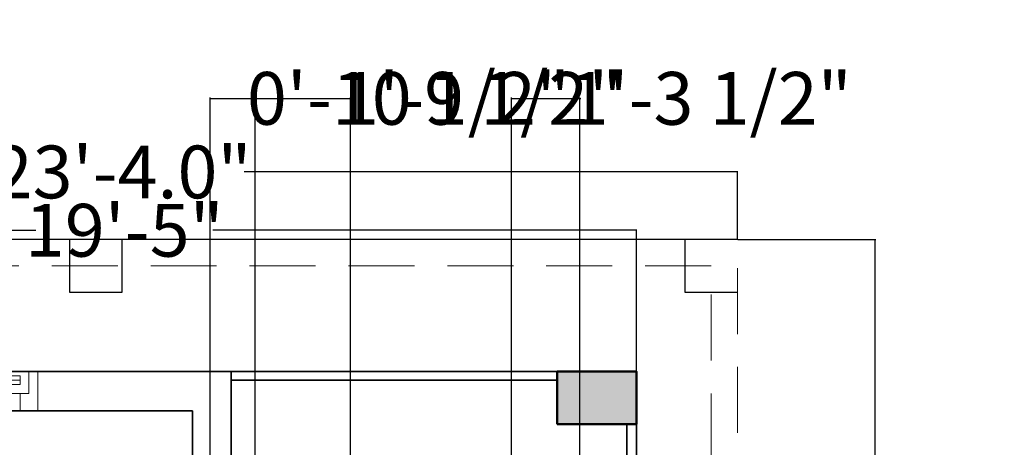
# Model space of a CAD drawing. Units: inches. Extents: x 1063 to 2718, y 423 to 1923.
# Tile 6 of 7: x 1268 to 1492, y 1038 to 1135. Entities that reach past the tile are written whole.
import ezdxf

# ---------------------------------------------------------------- set-up
doc = ezdxf.new("R2010")
doc.units = ezdxf.units.IN
doc.header["$LTSCALE"] = 6
doc.header["$MEASUREMENT"] = 0
doc.linetypes.add('HIDDEN', pattern=[0.375, 0.25, -0.125])
for name, color, linetype, lineweight in [('A-ANNO-DIMS', 2, 'Continuous', 18), ('A-COLS', 7, 'Continuous', 50), ('A-COLS-PATT', 252, 'Continuous', 13), ('A-GLAZ', 4, 'Continuous', 18), ('A-WALL', 7, 'Continuous', 35), ('C-PROP', 7, 'Continuous', 25), ('C-PROP-HIDN', 7, 'HIDDEN', 18)]:
    doc.layers.add(name, color=color, linetype=linetype, lineweight=lineweight)
doc.styles.get("Standard").update_dxf_attribs({"font": 'arial.ttf'})
doc.dimstyles.get("Standard").update_dxf_attribs({"dimtxt": 12, "dimasz": 0.18, "dimexe": 0.18, "dimexo": 0.0625, "dimgap": 0.09, "dimtad": 0, "dimtih": 1, "dimtoh": 1, "dimdec": 1, "dimzin": 0, "dimdsep": 46, "dimlunit": 3, "dimtxsty": 'Standard', "dimcen": 0.09, "dimadec": 0, "dimazin": 0, "dimtfac": 1, "dimtdec": 1, "dimtofl": 0, "dimtmove": 0, "dimatfit": 3, "dimfxl": 1, "dimtolj": 1, "dimtzin": 0, "dimarcsym": 0})

# ---------------------------------------------------------------- blocks, each defined once
blk = doc.blocks.new('*D5')
at = {"layer": 'A-ANNO-DIMS', "color": 0, "lineweight": -2, "ltscale": 6, "transparency": 16777216}
for p, q in [((1430.99, 1085.12), (1462.35, 1085.12)), ((1462.17, 1084.94), (1462.17, 1024.34)), ((1462.17, 951.3), (1462.17, 1011.9)), ((1430.99, 951.12), (1462.35, 951.12))]:
    blk.add_line(p, q, dxfattribs=at)
at = {"layer": 'A-ANNO-DIMS', "color": 0, "ltscale": 6, "transparency": 16777216}
for points in [[(1462.14, 1084.94), (1462.2, 1084.94), (1462.17, 1085.12)], [(1462.14, 951.3), (1462.2, 951.3), (1462.17, 951.12)]]:
    blk.add_solid(points, dxfattribs=at)
at = {"layer": 'Defpoints', "color": 0, "ltscale": 6, "transparency": 16777216}
for p in [(1430.93, 1085.12), (1462.17, 1085.12), (1430.93, 951.12)]:
    blk.add_point(p, dxfattribs=at)
at = {"layer": 'A-ANNO-DIMS', "color": 0, "ltscale": 6, "transparency": 16777216, "insert": (1462.17, 1018.12), "char_height": 12, "attachment_point": 5}
blk.add_mtext('\\A1;11\'-2.0"', dxfattribs=at)
blk = doc.blocks.new('*D6')
at = {"layer": 'A-ANNO-DIMS', "color": 0, "lineweight": -2, "ltscale": 6, "transparency": 16777216}
for p, q in [((1150.93, 1085.18), (1150.93, 1100.66)), ((1151.11, 1100.48), (1263.13, 1100.48)), ((1430.75, 1100.48), (1318.72, 1100.48)), ((1430.93, 1085.18), (1430.93, 1100.66))]:
    blk.add_line(p, q, dxfattribs=at)
at = {"layer": 'A-ANNO-DIMS', "color": 0, "ltscale": 6, "transparency": 16777216}
for points in [[(1151.11, 1100.51), (1151.11, 1100.45), (1150.93, 1100.48)], [(1430.75, 1100.51), (1430.75, 1100.45), (1430.93, 1100.48)]]:
    blk.add_solid(points, dxfattribs=at)
at = {"layer": 'Defpoints', "color": 0, "ltscale": 6, "transparency": 16777216}
for p in [(1430.93, 1100.48), (1150.93, 1085.12), (1430.93, 1085.12)]:
    blk.add_point(p, dxfattribs=at)
at = {"layer": 'A-ANNO-DIMS', "color": 0, "ltscale": 6, "transparency": 16777216, "insert": (1290.93, 1100.48), "char_height": 12, "attachment_point": 5}
blk.add_mtext('\\A1;23\'-4.0"', dxfattribs=at)
blk = doc.blocks.new('WIN-48-SLIDING')
at = {"ltscale": 6}
for p, q in [((0, 9), (4, 9)), ((4, 9), (4, 5)), ((48, 9), (44, 9)), ((44, 9), (44, 5)), ((4, 5), (2, 5)), ((2, 5), (2, 0)), ((4, 5), (44, 5)), ((4, 5), (6, 5)), ((6, 5), (6, 3)), ((44, 5), (42, 5)), ((42, 5), (42, 3)), ((44, 5), (46, 5)), ((46, 5), (46, 0)), ((6, 3), (4, 3)), ((4, 3), (4, 1)), ((42, 3), (44, 3)), ((44, 3), (44, 1)), ((4, 2), (44, 2)), ((4, 1), (6, 1)), ((6, 1), (6, 0)), ((44, 1), (42, 1)), ((42, 1), (42, 0)), ((48, 0), (0, 0)), ((2, 0), (46, 0))]:
    blk.add_line(p, q, dxfattribs=at)
blk.add_lwpolyline([(48, 0), (48, 9), (0, 9), (0, 0)], dxfattribs=at)
blk = doc.blocks.new('COLUMN-18X12')
blk.add_lwpolyline([(0, 0), (18, 0), (18, 12), (0, 12)], close=True)
blk = doc.blocks.new('PIER-12X12-CORNER')
blk.add_lwpolyline([(0, 0), (12, 0), (12, 12)])
blk = doc.blocks.new('PIER-12X12-INLINE')
blk.add_lwpolyline([(0, 0), (12, 0), (12, 12), (0, 12)])
blk = doc.blocks.new('*D44')
at = {"layer": 'A-ANNO-DIMS', "color": 0, "lineweight": -2, "ltscale": 6, "transparency": 16777216}
for p, q in [((1174.93, 1055.18), (1174.93, 1087.4)), ((1175.11, 1087.22), (1271.29, 1087.22)), ((1407.75, 1087.22), (1311.56, 1087.22)), ((1407.93, 1055.18), (1407.93, 1087.4))]:
    blk.add_line(p, q, dxfattribs=at)
at = {"layer": 'A-ANNO-DIMS', "color": 0, "ltscale": 6, "transparency": 16777216}
for points in [[(1175.11, 1087.25), (1175.11, 1087.19), (1174.93, 1087.22)], [(1407.75, 1087.25), (1407.75, 1087.19), (1407.93, 1087.22)]]:
    blk.add_solid(points, dxfattribs=at)
at = {"layer": 'Defpoints', "color": 0, "ltscale": 6, "transparency": 16777216}
for p in [(1407.93, 1087.22), (1174.93, 1055.12), (1407.93, 1055.12)]:
    blk.add_point(p, dxfattribs=at)
at = {"layer": 'A-ANNO-DIMS', "color": 0, "ltscale": 6, "transparency": 16777216, "insert": (1291.43, 1087.22), "char_height": 12, "attachment_point": 5}
blk.add_mtext('\\A1;19\'-5"', dxfattribs=at)
blk = doc.blocks.new('*D60')
at = {"layer": 'A-ANNO-DIMS', "color": 0, "lineweight": -2, "ltscale": 6, "transparency": 16777216}
for p, q in [((1321.21, 974.62), (1321.21, 1117.4)), ((1321.39, 1117.22), (1342.7, 1117.22)), ((1342.88, 974.62), (1342.88, 1117.4)), ((1342.88, 1117.22), (1343.06, 1117.22))]:
    blk.add_line(p, q, dxfattribs=at)
at = {"layer": 'A-ANNO-DIMS', "color": 0, "ltscale": 6, "transparency": 16777216}
for points in [[(1321.39, 1117.25), (1321.39, 1117.19), (1321.21, 1117.22)], [(1342.7, 1117.25), (1342.7, 1117.19), (1342.88, 1117.22)]]:
    blk.add_solid(points, dxfattribs=at)
at = {"layer": 'Defpoints', "color": 0, "ltscale": 6, "transparency": 16777216}
for p in [(1342.88, 1117.22), (1321.21, 974.55), (1342.88, 974.55)]:
    blk.add_point(p, dxfattribs=at)
at = {"layer": 'A-ANNO-DIMS', "color": 0, "ltscale": 6, "transparency": 16777216, "insert": (1372.52, 1117.22), "char_height": 12, "attachment_point": 5}
blk.add_mtext('\\A1;1\'-9 1/2"', dxfattribs=at)
blk = doc.blocks.new('*D62')
at = {"layer": 'A-ANNO-DIMS', "color": 0, "lineweight": -2, "ltscale": 6, "transparency": 16777216}
for p, q in [((1379.5, 974.73), (1379.5, 1117.4)), ((1379.68, 1117.22), (1394.9, 1117.22)), ((1395.08, 974.73), (1395.08, 1117.4)), ((1395.08, 1117.22), (1395.26, 1117.22))]:
    blk.add_line(p, q, dxfattribs=at)
at = {"layer": 'A-ANNO-DIMS', "color": 0, "ltscale": 6, "transparency": 16777216}
for points in [[(1379.68, 1117.25), (1379.68, 1117.19), (1379.5, 1117.22)], [(1394.9, 1117.25), (1394.9, 1117.19), (1395.08, 1117.22)]]:
    blk.add_solid(points, dxfattribs=at)
at = {"layer": 'Defpoints', "color": 0, "ltscale": 6, "transparency": 16777216}
for p in [(1395.08, 1117.22), (1379.5, 974.67), (1395.08, 974.67)]:
    blk.add_point(p, dxfattribs=at)
at = {"layer": 'A-ANNO-DIMS', "color": 0, "ltscale": 6, "transparency": 16777216, "insert": (1424.71, 1117.22), "char_height": 12, "attachment_point": 5}
blk.add_mtext('\\A1;1\'-3 1/2"', dxfattribs=at)
blk = doc.blocks.new('*D64')
at = {"layer": 'A-ANNO-DIMS', "color": 0, "lineweight": -2, "ltscale": 6, "transparency": 16777216}
for p, q in [((1310.93, 978.18), (1310.93, 1117.4)), ((1311.11, 1117.22), (1321.03, 1117.22)), ((1321.21, 974.62), (1321.21, 1117.4)), ((1321.21, 1117.22), (1321.39, 1117.22))]:
    blk.add_line(p, q, dxfattribs=at)
at = {"layer": 'A-ANNO-DIMS', "color": 0, "ltscale": 6, "transparency": 16777216}
for points in [[(1311.11, 1117.25), (1311.11, 1117.19), (1310.93, 1117.22)], [(1321.03, 1117.25), (1321.03, 1117.19), (1321.21, 1117.22)]]:
    blk.add_solid(points, dxfattribs=at)
at = {"layer": 'Defpoints', "color": 0, "ltscale": 6, "transparency": 16777216}
for p in [(1321.21, 1117.22), (1310.93, 978.12), (1321.21, 974.55)]:
    blk.add_point(p, dxfattribs=at)
at = {"layer": 'A-ANNO-DIMS', "color": 0, "ltscale": 6, "transparency": 16777216, "insert": (1356.07, 1117.22), "char_height": 12, "attachment_point": 5}
blk.add_mtext('\\A1;0\'-10 1/2"', dxfattribs=at)

msp = doc.modelspace()

# ---------------------------------------------------------------- hatches: boundary and pattern name
at = {"layer": 'A-COLS-PATT', "ltscale": 6}
h = msp.add_hatch(color=256, dxfattribs=at)
h.dxf.hatch_style = 1
h.paths.add_polyline_path([(1192.93, 603.12), (1174.93, 603.12), (1174.93, 591.12), (1192.93, 591.12)])
h.paths.add_polyline_path([(1407.93, 603.12), (1389.93, 603.12), (1389.93, 591.12), (1407.93, 591.12)])
h.paths.add_polyline_path([(1192.93, 756.12), (1174.93, 756.12), (1174.93, 744.12), (1192.93, 744.12)])
h.paths.add_polyline_path([(1407.93, 761.11), (1389.93, 761.11), (1389.93, 749.11), (1407.93, 749.11)])
h.paths.add_polyline_path([(1455.93, 761.11), (1437.93, 761.11), (1437.93, 749.11), (1455.93, 749.11)])
h.paths.add_polyline_path([(1455.93, 910.12), (1437.93, 910.12), (1437.93, 898.12), (1455.93, 898.12)])
h.paths.add_polyline_path([(1407.93, 910.12), (1389.93, 910.12), (1389.93, 898.12), (1407.93, 898.12)])
h.paths.add_polyline_path([(1192.93, 910.12), (1174.93, 910.12), (1174.93, 898.12), (1192.93, 898.12)])
h.paths.add_polyline_path([(1192.93, 1055.12), (1174.93, 1055.12), (1174.93, 1043.12), (1192.93, 1043.12)])
h.paths.add_polyline_path([(1407.93, 1055.12), (1389.93, 1055.12), (1389.93, 1043.12), (1407.93, 1043.12)])

# ---------------------------------------------------------------- linework, layer by layer
at = {"layer": 'A-WALL'}
for p, q in [((1407.93, 1055.12), (1174.93, 1055.12)), ((1315.75, 1055.12), (1315.75, 987.12)), ((1315.75, 1053.12), (1389.93, 1053.12)), ((1306.93, 1046.12), (1192.93, 1046.12)), ((1306.93, 1046.12), (1306.93, 902.12)), ((1405.75, 1043.12), (1405.75, 987.12))]:
    msp.add_line(p, q, dxfattribs=at)
at = {"layer": 'A-WALL', "ltscale": 6}
msp.add_line((1407.93, 1055.12), (1407.93, 591.12), dxfattribs=at)
at = {"layer": 'C-PROP'}
msp.add_line((1430.93, 1085.12), (1150.93, 1085.12), dxfattribs=at)
at = {"layer": 'C-PROP-HIDN', "ltscale": 10}
for p, q in [((1430.93, 951.12), (1430.93, 1085.12)), ((1424.93, 1079.12), (1156.93, 1079.12)), ((1424.93, 945.12), (1424.93, 1079.12))]:
    msp.add_line(p, q, dxfattribs=at)

# ---------------------------------------------------------------- block references
at = {"layer": 'A-COLS'}
msp.add_blockref('COLUMN-18X12', (1389.93, 1043.12), dxfattribs=at)
at = {"layer": 'A-GLAZ', "rotation": 180}
msp.add_blockref('WIN-48-SLIDING', (1271.72, 1055.12), dxfattribs=at)
at = {"layer": 'C-PROP', "rotation": 270}
for name, p in [('PIER-12X12-INLINE', (1278.93, 1085.12)), ('PIER-12X12-CORNER', (1418.93, 1085.12))]:
    msp.add_blockref(name, p, dxfattribs=at)

# ---------------------------------------------------------------- dimensions: what is measured, and where the dimension line sits
at = {"layer": 'A-ANNO-DIMS', "ltscale": 6}
for base, p1, p2, override, picture, middle in [((1321.21, 1117.22), (1310.93, 978.12), (1321.21, 974.55), {"dimdec": 1, "dimlfac": 1, "dimrnd": 0, "dimzin": 1, "dimdsep": 46, "dimlunit": 4, "dimfrac": 2}, '*D64', (1356.07, 1117.22)), ((1342.88, 1117.22), (1321.21, 974.55), (1342.88, 974.55), {"dimdec": 1, "dimlfac": 1, "dimrnd": 0, "dimzin": 1, "dimdsep": 46, "dimlunit": 4, "dimfrac": 2}, '*D60', (1372.52, 1117.22)), ((1395.08, 1117.22), (1379.5, 974.67), (1395.08, 974.67), {"dimdec": 1, "dimlfac": 1, "dimrnd": 0, "dimzin": 1, "dimdsep": 46, "dimlunit": 4, "dimfrac": 2}, '*D62', (1424.71, 1117.22)), ((1430.93, 1100.48), (1150.93, 1085.12), (1430.93, 1085.12), {"dimclrd": 0, "dimclre": 0, "dimclrt": 0}, '*D6', (1290.93, 1100.48)), ((1407.93, 1087.22), (1174.93, 1055.12), (1407.93, 1055.12), {"dimdec": 1, "dimlfac": 1, "dimrnd": 0, "dimzin": 1, "dimdsep": 46, "dimlunit": 4, "dimfrac": 2}, '*D44', (1291.43, 1087.22))]:
    dim = msp.add_linear_dim(base=base, p1=p1, p2=p2, dimstyle='Standard', override=override, dxfattribs=at)
    dim.commit()
    dim.dimension.update_dxf_attribs({"geometry": picture, "text_midpoint": middle})
dim = msp.add_linear_dim(base=(1462.17, 1085.12), p1=(1430.93, 951.12), p2=(1430.93, 1085.12), angle=90, dimstyle='Standard', override={"dimclrd": 0, "dimclre": 0, "dimclrt": 0}, dxfattribs=at)
dim.commit()
dim.dimension.update_dxf_attribs({"geometry": '*D5', "text_midpoint": (1462.17, 1018.12)})

doc.saveas('drawing.dxf')
